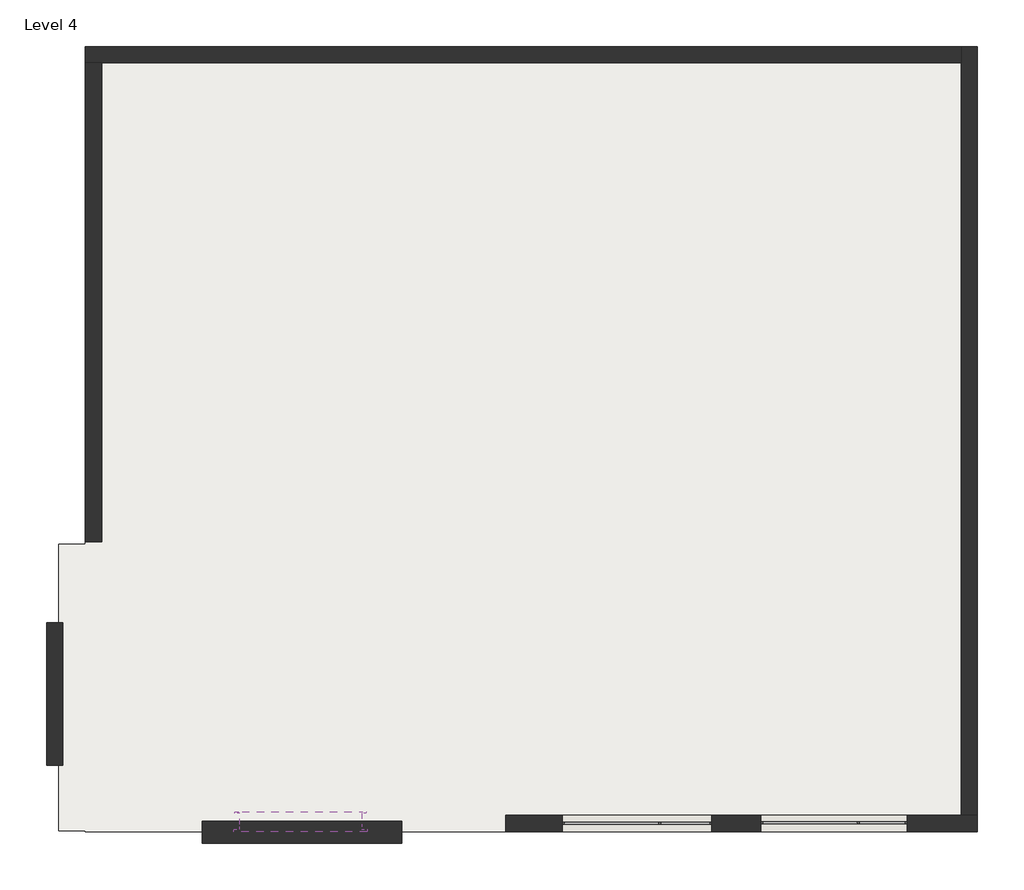
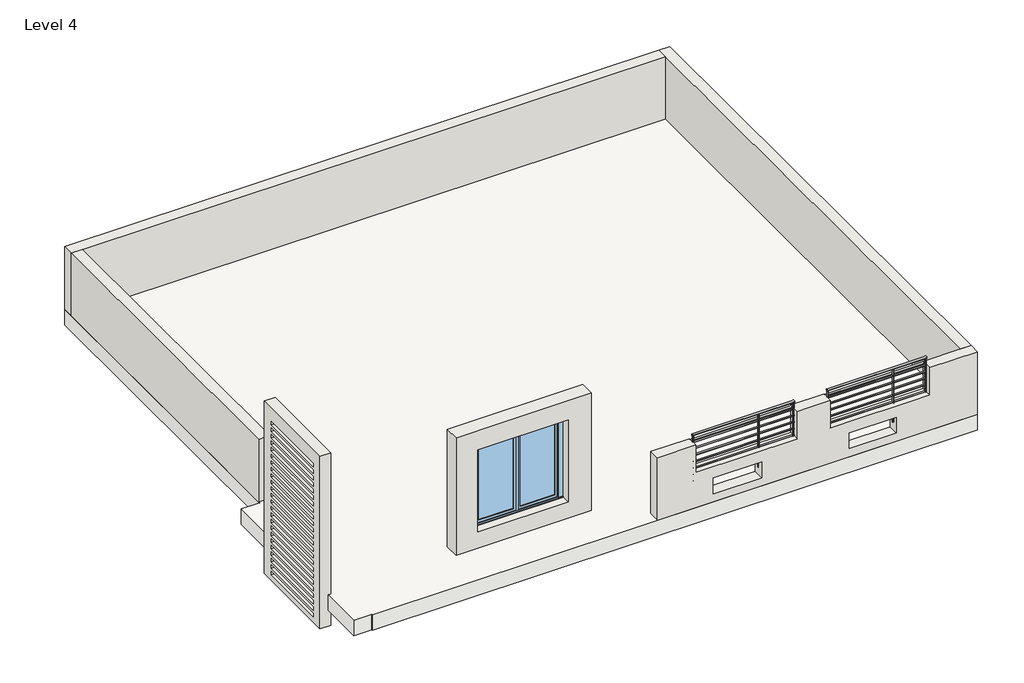
# One storey: 6 walls, 2 railings, 1 roof, 1 window.
"""IFC4 building model written with IfcOpenShell, lengths in millimetres."""

from ifc_helpers import new_model, si_unit, point, frame, frame_2d, origin, place, context, project, spatial, polyline, circle_curve, trimmed, segment, composite_curve, outline, extrude, faceted_brep, transform, mapped, element, save
from components import walls_2_walls_1_3adabfa7, window_514a67b1

model = new_model("IFC4")

# Units and contexts
model_context = context("Model", 3, world=origin())
ifc_project = project(units=[si_unit("LENGTHUNIT", "METRE", prefix="MILLI")], contexts=[model_context])

# Site, building, storey
site = spatial("IfcSite", under=ifc_project)
building = spatial("IfcBuilding", under=site)
storey = spatial("IfcBuildingStorey", under=building, Name="Level 4", Elevation=10972.8)

# Railings
placement = place(None, origin())
element("IfcRailing", 1, ObjectType="Guardrail - Pipe", at=placement, inside=storey, context=model_context, shape_type="SweptSolid", body=[
    extrude(outline(composite_curve([segment(trimmed(circle_curve(frame_2d((1736.4093308, 12477.75)), 19.05), [point((1717.3593308, 12477.75))], [point((1755.4593308, 12477.75))], False, "CARTESIAN"), True, "CONTINUOUS"), segment(trimmed(circle_curve(frame_2d((1736.4093308, 12477.75)), 19.05), [point((1755.4593308, 12477.75))], [point((1717.3593308, 12477.75))], False, "CARTESIAN"), True, "CONTINUOUS")], self_intersect=False)), frame((-4064.538951, 0.0, 0.0), z_axis=(1.0, 0.0, 0.0), x_axis=(0.0, 1.0, 0.0)), (0.0, 0.0, 1.0), 1872.0501462),
    extrude(outline(composite_curve([segment(trimmed(circle_curve(frame_2d((1660.2093308, 12630.15)), 19.05), [point((1641.1593308, 12630.15))], [point((1679.2593308, 12630.15))], False, "CARTESIAN"), True, "CONTINUOUS"), segment(trimmed(circle_curve(frame_2d((1660.2093308, 12630.15)), 19.05), [point((1679.2593308, 12630.15))], [point((1641.1593308, 12630.15))], False, "CARTESIAN"), True, "CONTINUOUS")], self_intersect=False)), frame((-4064.538951, 0.0, 0.0), z_axis=(1.0, 0.0, 0.0), x_axis=(0.0, 1.0, 0.0)), (0.0, 0.0, 1.0), 1872.0501462),
    extrude(outline(composite_curve([segment(trimmed(circle_curve(frame_2d((1660.2093308, 12484.1)), 12.7), [point((1672.9093308, 12484.1))], [point((1647.5093308, 12484.1))], False, "CARTESIAN"), True, "CONTINUOUS"), segment(trimmed(circle_curve(frame_2d((1660.2093308, 12484.1)), 12.7), [point((1647.5093308, 12484.1))], [point((1672.9093308, 12484.1))], False, "CARTESIAN"), True, "CONTINUOUS")], self_intersect=False)), frame((-4064.538951, 0.0, 0.0), z_axis=(1.0, 0.0, 0.0), x_axis=(0.0, 1.0, 0.0)), (0.0, 0.0, 1.0), 1872.0501462),
    extrude(outline(composite_curve([segment(trimmed(circle_curve(frame_2d((1660.2093308, 12357.1)), 12.7), [point((1672.9093308, 12357.1))], [point((1647.5093308, 12357.1))], False, "CARTESIAN"), True, "CONTINUOUS"), segment(trimmed(circle_curve(frame_2d((1660.2093308, 12357.1)), 12.7), [point((1647.5093308, 12357.1))], [point((1672.9093308, 12357.1))], False, "CARTESIAN"), True, "CONTINUOUS")], self_intersect=False)), frame((-4064.538951, 0.0, 0.0), z_axis=(1.0, 0.0, 0.0), x_axis=(0.0, 1.0, 0.0)), (0.0, 0.0, 1.0), 1872.0501462),
    extrude(outline(composite_curve([segment(trimmed(circle_curve(frame_2d((1660.2093308, 12230.1)), 12.7), [point((1672.9093308, 12230.1))], [point((1647.5093308, 12230.1))], False, "CARTESIAN"), True, "CONTINUOUS"), segment(trimmed(circle_curve(frame_2d((1660.2093308, 12230.1)), 12.7), [point((1647.5093308, 12230.1))], [point((1672.9093308, 12230.1))], False, "CARTESIAN"), True, "CONTINUOUS")], self_intersect=False)), frame((-4064.538951, 0.0, 0.0), z_axis=(1.0, 0.0, 0.0), x_axis=(0.0, 1.0, 0.0)), (0.0, 0.0, 1.0), 1872.0501462),
    extrude(outline(composite_curve([segment(trimmed(circle_curve(frame_2d((1660.2093308, 12103.1)), 12.7), [point((1672.9093308, 12103.1))], [point((1647.5093308, 12103.1))], False, "CARTESIAN"), True, "CONTINUOUS"), segment(trimmed(circle_curve(frame_2d((1660.2093308, 12103.1)), 12.7), [point((1647.5093308, 12103.1))], [point((1672.9093308, 12103.1))], False, "CARTESIAN"), True, "CONTINUOUS")], self_intersect=False)), frame((-4064.538951, 0.0, 0.0), z_axis=(1.0, 0.0, 0.0), x_axis=(0.0, 1.0, 0.0)), (0.0, 0.0, 1.0), 1872.0501462),
    extrude(outline(composite_curve([segment(trimmed(circle_curve(frame_2d((1660.2093308, 11976.1)), 12.7), [point((1672.9093308, 11976.1))], [point((1647.5093308, 11976.1))], False, "CARTESIAN"), True, "CONTINUOUS"), segment(trimmed(circle_curve(frame_2d((1660.2093308, 11976.1)), 12.7), [point((1647.5093308, 11976.1))], [point((1672.9093308, 11976.1))], False, "CARTESIAN"), True, "CONTINUOUS")], self_intersect=False)), frame((-4064.538951, 0.0, 0.0), z_axis=(1.0, 0.0, 0.0), x_axis=(0.0, 1.0, 0.0)), (0.0, 0.0, 1.0), 1872.0501462),
    extrude(outline(composite_curve([segment(trimmed(circle_curve(frame_2d((1660.2093308, 11849.1)), 12.7), [point((1672.9093308, 11849.1))], [point((1647.5093308, 11849.1))], False, "CARTESIAN"), True, "CONTINUOUS"), segment(trimmed(circle_curve(frame_2d((1660.2093308, 11849.1)), 12.7), [point((1647.5093308, 11849.1))], [point((1672.9093308, 11849.1))], False, "CARTESIAN"), True, "CONTINUOUS")], self_intersect=False)), frame((-4064.538951, 0.0, 0.0), z_axis=(1.0, 0.0, 0.0), x_axis=(0.0, 1.0, 0.0)), (0.0, 0.0, 1.0), 1872.0501462),
    extrude(outline(composite_curve([segment(trimmed(circle_curve(frame_2d((1660.2093308, 11722.1)), 12.7), [point((1672.9093308, 11722.1))], [point((1647.5093308, 11722.1))], False, "CARTESIAN"), True, "CONTINUOUS"), segment(trimmed(circle_curve(frame_2d((1660.2093308, 11722.1)), 12.7), [point((1647.5093308, 11722.1))], [point((1672.9093308, 11722.1))], False, "CARTESIAN"), True, "CONTINUOUS")], self_intersect=False)), frame((-4064.538951, 0.0, 0.0), z_axis=(1.0, 0.0, 0.0), x_axis=(0.0, 1.0, 0.0)), (0.0, 0.0, 1.0), 1872.0501462),
    extrude(outline(composite_curve([segment(trimmed(circle_curve(frame_2d((-2845.338951, 1660.2093308)), 12.7), [point((-2845.338951, 1672.9093308))], [point((-2845.338951, 1647.5093308))], False, "CARTESIAN"), True, "CONTINUOUS"), segment(trimmed(circle_curve(frame_2d((-2845.338951, 1660.2093308)), 12.7), [point((-2845.338951, 1647.5093308))], [point((-2845.338951, 1672.9093308))], False, "CARTESIAN"), True, "CONTINUOUS")], self_intersect=False)), frame((0.0, 0.0, 11582.4), z_axis=(0.0, 0.0, 1.0), x_axis=(1.0, 0.0, 0.0)), (0.0, 0.0, 1.0), 1028.7),
    extrude(outline(composite_curve([segment(trimmed(circle_curve(frame_2d((-2205.1888049, 1660.2093308)), 12.7), [point((-2205.1888049, 1672.9093308))], [point((-2205.1888049, 1647.5093308))], False, "CARTESIAN"), True, "CONTINUOUS"), segment(trimmed(circle_curve(frame_2d((-2205.1888049, 1660.2093308)), 12.7), [point((-2205.1888049, 1647.5093308))], [point((-2205.1888049, 1672.9093308))], False, "CARTESIAN"), True, "CONTINUOUS")], self_intersect=False)), frame((0.0, 0.0, 11582.4), z_axis=(0.0, 0.0, 1.0), x_axis=(1.0, 0.0, 0.0)), (0.0, 0.0, 1.0), 1028.7),
    extrude(outline(composite_curve([segment(trimmed(circle_curve(frame_2d((-4051.838951, 1660.2093308)), 12.7), [point((-4051.838951, 1672.9093308))], [point((-4051.838951, 1647.5093308))], False, "CARTESIAN"), True, "CONTINUOUS"), segment(trimmed(circle_curve(frame_2d((-4051.838951, 1660.2093308)), 12.7), [point((-4051.838951, 1647.5093308))], [point((-4051.838951, 1672.9093308))], False, "CARTESIAN"), True, "CONTINUOUS")], self_intersect=False)), frame((0.0, 0.0, 11582.4), z_axis=(0.0, 0.0, 1.0), x_axis=(1.0, 0.0, 0.0)), (0.0, 0.0, 1.0), 1028.7),
])
element("IfcRailing", 2, ObjectType="Guardrail - Pipe", at=placement, inside=storey, context=model_context, shape_type="SweptSolid", body=[
    extrude(outline(composite_curve([segment(trimmed(circle_curve(frame_2d((1742.0864664, 12477.75)), 19.05), [point((1723.0364664, 12477.75))], [point((1761.1364664, 12477.75))], False, "CARTESIAN"), True, "CONTINUOUS"), segment(trimmed(circle_curve(frame_2d((1742.0864664, 12477.75)), 19.05), [point((1761.1364664, 12477.75))], [point((1723.0364664, 12477.75))], False, "CARTESIAN"), True, "CONTINUOUS")], self_intersect=False)), frame((-1582.8888049, 0.0, 0.0), z_axis=(1.0, 0.0, 0.0), x_axis=(0.0, 1.0, 0.0)), (0.0, 0.0, 1.0), 1827.3417832),
    extrude(outline(composite_curve([segment(trimmed(circle_curve(frame_2d((1665.8864664, 12630.15)), 19.05), [point((1646.8364664, 12630.15))], [point((1684.9364664, 12630.15))], False, "CARTESIAN"), True, "CONTINUOUS"), segment(trimmed(circle_curve(frame_2d((1665.8864664, 12630.15)), 19.05), [point((1684.9364664, 12630.15))], [point((1646.8364664, 12630.15))], False, "CARTESIAN"), True, "CONTINUOUS")], self_intersect=False)), frame((-1582.8888049, 0.0, 0.0), z_axis=(1.0, 0.0, 0.0), x_axis=(0.0, 1.0, 0.0)), (0.0, 0.0, 1.0), 1827.3417832),
    extrude(outline(composite_curve([segment(trimmed(circle_curve(frame_2d((1665.8864664, 12484.1)), 12.7), [point((1678.5864664, 12484.1))], [point((1653.1864664, 12484.1))], False, "CARTESIAN"), True, "CONTINUOUS"), segment(trimmed(circle_curve(frame_2d((1665.8864664, 12484.1)), 12.7), [point((1653.1864664, 12484.1))], [point((1678.5864664, 12484.1))], False, "CARTESIAN"), True, "CONTINUOUS")], self_intersect=False)), frame((-1582.8888049, 0.0, 0.0), z_axis=(1.0, 0.0, 0.0), x_axis=(0.0, 1.0, 0.0)), (0.0, 0.0, 1.0), 1827.3417832),
    extrude(outline(composite_curve([segment(trimmed(circle_curve(frame_2d((1665.8864664, 12357.1)), 12.7), [point((1678.5864664, 12357.1))], [point((1653.1864664, 12357.1))], False, "CARTESIAN"), True, "CONTINUOUS"), segment(trimmed(circle_curve(frame_2d((1665.8864664, 12357.1)), 12.7), [point((1653.1864664, 12357.1))], [point((1678.5864664, 12357.1))], False, "CARTESIAN"), True, "CONTINUOUS")], self_intersect=False)), frame((-1582.8888049, 0.0, 0.0), z_axis=(1.0, 0.0, 0.0), x_axis=(0.0, 1.0, 0.0)), (0.0, 0.0, 1.0), 1827.3417832),
    extrude(outline(composite_curve([segment(trimmed(circle_curve(frame_2d((1665.8864664, 12230.1)), 12.7), [point((1678.5864664, 12230.1))], [point((1653.1864664, 12230.1))], False, "CARTESIAN"), True, "CONTINUOUS"), segment(trimmed(circle_curve(frame_2d((1665.8864664, 12230.1)), 12.7), [point((1653.1864664, 12230.1))], [point((1678.5864664, 12230.1))], False, "CARTESIAN"), True, "CONTINUOUS")], self_intersect=False)), frame((-1582.8888049, 0.0, 0.0), z_axis=(1.0, 0.0, 0.0), x_axis=(0.0, 1.0, 0.0)), (0.0, 0.0, 1.0), 1827.3417832),
    extrude(outline(composite_curve([segment(trimmed(circle_curve(frame_2d((1665.8864664, 12103.1)), 12.7), [point((1678.5864664, 12103.1))], [point((1653.1864664, 12103.1))], False, "CARTESIAN"), True, "CONTINUOUS"), segment(trimmed(circle_curve(frame_2d((1665.8864664, 12103.1)), 12.7), [point((1653.1864664, 12103.1))], [point((1678.5864664, 12103.1))], False, "CARTESIAN"), True, "CONTINUOUS")], self_intersect=False)), frame((-1582.8888049, 0.0, 0.0), z_axis=(1.0, 0.0, 0.0), x_axis=(0.0, 1.0, 0.0)), (0.0, 0.0, 1.0), 1827.3417832),
    extrude(outline(composite_curve([segment(trimmed(circle_curve(frame_2d((1665.8864664, 11976.1)), 12.7), [point((1678.5864664, 11976.1))], [point((1653.1864664, 11976.1))], False, "CARTESIAN"), True, "CONTINUOUS"), segment(trimmed(circle_curve(frame_2d((1665.8864664, 11976.1)), 12.7), [point((1653.1864664, 11976.1))], [point((1678.5864664, 11976.1))], False, "CARTESIAN"), True, "CONTINUOUS")], self_intersect=False)), frame((-1582.8888049, 0.0, 0.0), z_axis=(1.0, 0.0, 0.0), x_axis=(0.0, 1.0, 0.0)), (0.0, 0.0, 1.0), 1827.3417832),
    extrude(outline(composite_curve([segment(trimmed(circle_curve(frame_2d((1665.8864664, 11849.1)), 12.7), [point((1678.5864664, 11849.1))], [point((1653.1864664, 11849.1))], False, "CARTESIAN"), True, "CONTINUOUS"), segment(trimmed(circle_curve(frame_2d((1665.8864664, 11849.1)), 12.7), [point((1653.1864664, 11849.1))], [point((1678.5864664, 11849.1))], False, "CARTESIAN"), True, "CONTINUOUS")], self_intersect=False)), frame((-1582.8888049, 0.0, 0.0), z_axis=(1.0, 0.0, 0.0), x_axis=(0.0, 1.0, 0.0)), (0.0, 0.0, 1.0), 1827.3417832),
    extrude(outline(composite_curve([segment(trimmed(circle_curve(frame_2d((1665.8864664, 11722.1)), 12.7), [point((1678.5864664, 11722.1))], [point((1653.1864664, 11722.1))], False, "CARTESIAN"), True, "CONTINUOUS"), segment(trimmed(circle_curve(frame_2d((1665.8864664, 11722.1)), 12.7), [point((1653.1864664, 11722.1))], [point((1678.5864664, 11722.1))], False, "CARTESIAN"), True, "CONTINUOUS")], self_intersect=False)), frame((-1582.8888049, 0.0, 0.0), z_axis=(1.0, 0.0, 0.0), x_axis=(0.0, 1.0, 0.0)), (0.0, 0.0, 1.0), 1827.3417832),
    extrude(outline(composite_curve([segment(trimmed(circle_curve(frame_2d((-363.6888049, 1665.8864664)), 12.7), [point((-363.6888049, 1678.5864664))], [point((-363.6888049, 1653.1864664))], False, "CARTESIAN"), True, "CONTINUOUS"), segment(trimmed(circle_curve(frame_2d((-363.6888049, 1665.8864664)), 12.7), [point((-363.6888049, 1653.1864664))], [point((-363.6888049, 1678.5864664))], False, "CARTESIAN"), True, "CONTINUOUS")], self_intersect=False)), frame((0.0, 0.0, 11582.4), z_axis=(0.0, 0.0, 1.0), x_axis=(1.0, 0.0, 0.0)), (0.0, 0.0, 1.0), 1028.7),
    extrude(outline(composite_curve([segment(trimmed(circle_curve(frame_2d((231.7529784, 1665.8864664)), 12.7), [point((231.7529784, 1678.5864664))], [point((231.7529784, 1653.1864664))], False, "CARTESIAN"), True, "CONTINUOUS"), segment(trimmed(circle_curve(frame_2d((231.7529784, 1665.8864664)), 12.7), [point((231.7529784, 1653.1864664))], [point((231.7529784, 1678.5864664))], False, "CARTESIAN"), True, "CONTINUOUS")], self_intersect=False)), frame((0.0, 0.0, 11582.4), z_axis=(0.0, 0.0, 1.0), x_axis=(1.0, 0.0, 0.0)), (0.0, 0.0, 1.0), 1028.7),
    extrude(outline(composite_curve([segment(trimmed(circle_curve(frame_2d((-1570.1888049, 1665.8864664)), 12.7), [point((-1570.1888049, 1678.5864664))], [point((-1570.1888049, 1653.1864664))], False, "CARTESIAN"), True, "CONTINUOUS"), segment(trimmed(circle_curve(frame_2d((-1570.1888049, 1665.8864664)), 12.7), [point((-1570.1888049, 1653.1864664))], [point((-1570.1888049, 1678.5864664))], False, "CARTESIAN"), True, "CONTINUOUS")], self_intersect=False)), frame((0.0, 0.0, 11582.4), z_axis=(0.0, 0.0, 1.0), x_axis=(1.0, 0.0, 0.0)), (0.0, 0.0, 1.0), 1028.7),
])

# Roof
element("IfcRoof", 3, ObjectType="Generic - 12\"", at=placement, inside=storey, context=model_context, shape_type="SweptSolid", body=[
    extrude(outline(polyline([(-10018.4747472, 11358.0609482), (1122.6002528, 11358.0609482), (1122.6002528, 1553.6609482), (-10019.8638097, 1553.6609482), (-10019.8638097, 1567.9484482), (-10352.5857575, 1567.9484482), (-10352.5857575, 5144.9959854), (-10018.4747472, 5144.9959854), (-10018.4747472, 11358.0609482)])), frame((0.0, 0.0, 10972.8), z_axis=(0.0, 0.0, 1.0), x_axis=(1.0, 0.0, 0.0)), (0.0, 0.0, 1.0), 304.8),
])

# Walls
element("IfcWall", 4, ObjectType="Generic - 8\"", at=placement, inside=storey, context=model_context, shape_type="Brep", body=[
    faceted_brep([(-4770.1997472, 1553.6609482, 11277.6), (1122.6002528, 1553.6609482, 11277.6), (1122.6002528, 1553.6609482, 11963.4), (1122.6002528, 1553.6609482, 12496.8), (244.4529784, 1553.6609482, 12496.8), (244.4529784, 1553.6609482, 11963.4), (-1582.8888049, 1553.6609482, 11963.4), (-1582.8888049, 1553.6609482, 12496.8), (-2192.4888049, 1553.6609482, 12496.8), (-2192.4888049, 1553.6609482, 11963.4), (-4064.538951, 1553.6609482, 11963.4), (-4064.538951, 1553.6609482, 12496.8), (-4770.1997472, 1553.6609482, 12496.8), (-2852.1449663, 1553.6609482, 11741.1892952), (-2852.1449663, 1553.6609482, 11436.3892952), (-3741.1449663, 1553.6609482, 11436.3892952), (-3741.1449663, 1553.6609482, 11741.1892952), (-369.8611252, 1553.6609482, 11741.1892952), (-369.8611252, 1553.6609482, 11436.3892952), (-1235.0084685, 1553.6609482, 11436.3892952), (-1235.0084685, 1553.6609482, 11741.1892952), (-4770.1997472, 1756.8609482, 11277.6), (-4770.1997472, 1756.8609482, 12496.8), (-4064.538951, 1756.8609482, 12496.8), (-4064.538951, 1756.8609482, 11963.4), (-2192.4888049, 1756.8609482, 11963.4), (-2192.4888049, 1756.8609482, 12496.8), (-1582.8888049, 1756.8609482, 12496.8), (-1582.8888049, 1756.8609482, 11963.4), (244.4529784, 1756.8609482, 11963.4), (244.4529784, 1756.8609482, 12496.8), (919.4002528, 1756.8609482, 12496.8), (1122.6002528, 1756.8609482, 12496.8), (1122.6002528, 1756.8609482, 11963.4), (1122.6002528, 1756.8609482, 11277.6), (919.4002528, 1756.8609482, 11277.6), (-2852.1449663, 1756.8609482, 11741.1892952), (-3741.1449663, 1756.8609482, 11741.1892952), (-3741.1449663, 1756.8609482, 11436.3892952), (-2852.1449663, 1756.8609482, 11436.3892952), (-369.8611252, 1756.8609482, 11741.1892952), (-1235.0084685, 1756.8609482, 11741.1892952), (-1235.0084685, 1756.8609482, 11436.3892952), (-369.8611252, 1756.8609482, 11436.3892952)], [[[0, 1, 2, 3, 4, 5, 6, 7, 8, 9, 10, 11, 12], [13, 14, 15, 16], [17, 18, 19, 20]], [[21, 22, 23, 24, 25, 26, 27, 28, 29, 30, 31, 32, 33, 34, 35], [36, 37, 38, 39], [40, 41, 42, 43]], [[1, 0, 21, 35, 34]], [[0, 12, 22, 21]], [[6, 5, 29, 28]], [[7, 6, 28, 27]], [[8, 7, 27, 26]], [[9, 8, 26, 25]], [[10, 9, 25, 24]], [[14, 13, 36, 39]], [[15, 14, 39, 38]], [[16, 15, 38, 37]], [[13, 16, 37, 36]], [[18, 17, 40, 43]], [[19, 18, 43, 42]], [[20, 19, 42, 41]], [[17, 20, 41, 40]], [[4, 3, 32, 31, 30]], [[5, 4, 30, 29]], [[11, 10, 24, 23]], [[12, 11, 23, 22]], [[3, 2, 1, 34, 33, 32]]]),
])
element("IfcWall", 5, ObjectType="Generic - 8\"", at=placement, inside=storey, context=model_context, shape_type="Brep", body=[
    faceted_brep([(1122.6002528, 1756.8609482, 11277.6), (1122.6002528, 11358.0609482, 11277.6), (1122.6002528, 11358.0609482, 12496.8), (1122.6002528, 1756.8609482, 12496.8), (919.4002528, 1756.8609482, 11277.6), (919.4002528, 1756.8609482, 12496.8), (919.4002528, 11154.8609482, 12496.8), (919.4002528, 11358.0609482, 12496.8), (919.4002528, 11358.0609482, 11277.6), (919.4002528, 11154.8609482, 11277.6)], [[[0, 1, 2, 3]], [[4, 5, 6, 7, 8, 9]], [[1, 0, 4, 9, 8]], [[3, 2, 7, 6, 5]], [[0, 3, 5, 4]], [[2, 1, 8, 7]]]),
])
element("IfcWall", 6, ObjectType="Generic - 8\"", at=placement, inside=storey, context=model_context, shape_type="Brep", body=[
    faceted_brep([(919.4002528, 11358.0609482, 11277.6), (-10018.4747472, 11358.0609482, 11277.6), (-10018.4747472, 11358.0609482, 12496.8), (919.4002528, 11358.0609482, 12496.8), (919.4002528, 11154.8609482, 11277.6), (919.4002528, 11154.8609482, 12496.8), (-9815.2747472, 11154.8609482, 12496.8), (-10018.4747472, 11154.8609482, 12496.8), (-10018.4747472, 11154.8609482, 11277.6), (-9815.2747472, 11154.8609482, 11277.6)], [[[0, 1, 2, 3]], [[4, 5, 6, 7, 8, 9]], [[1, 0, 4, 9, 8]], [[3, 2, 7, 6, 5]], [[0, 3, 5, 4]], [[2, 1, 8, 7]]]),
])
element("IfcWall", 7, ObjectType="Generic - 8\"", at=placement, inside=storey, context=model_context, shape_type="Brep", body=[
    faceted_brep([(-10018.4747472, 11154.8609482, 11277.6), (-10018.4747472, 5306.9209854, 11277.6), (-10018.4747472, 5179.9209854, 11277.6), (-10018.4747472, 5174.7484482, 11277.6), (-10018.4747472, 5174.7484482, 12496.8), (-10018.4747472, 11154.8609482, 12496.8), (-9815.2747472, 11154.8609482, 11277.6), (-9815.2747472, 11154.8609482, 12496.8), (-9815.2747472, 5174.7484482, 12496.8), (-9815.2747472, 5174.7484482, 11277.6)], [[[0, 1, 2, 3, 4, 5]], [[6, 7, 8, 9]], [[3, 2, 1, 0, 6, 9]], [[5, 4, 8, 7]], [[0, 5, 7, 6]], [[4, 3, 9, 8]]]),
])
element("IfcWall", 8, ObjectType="Generic - 8\"", at=placement, inside=storey, context=model_context, shape_type="SweptSolid", body=[
    extrude(outline(polyline([(4162.4454783, 10668.0), (2382.8579783, 10668.0), (2382.8579783, 14023.1950228), (4162.4454783, 14023.1950228), (4162.4454783, 10668.0)]), holes=[polyline([(3937.4533381, 13762.2542182), (2591.2533381, 13762.2542182), (2591.2533381, 13698.7542182), (3937.4533381, 13698.7542182), (3937.4533381, 13762.2542182)]), polyline([(3937.4533381, 13635.2542182), (2591.2533381, 13635.2542182), (2591.2533381, 13571.7542182), (3937.4533381, 13571.7542182), (3937.4533381, 13635.2542182)]), polyline([(3937.4533381, 13508.2542182), (2591.2533381, 13508.2542182), (2591.2533381, 13444.7542182), (3937.4533381, 13444.7542182), (3937.4533381, 13508.2542182)]), polyline([(3937.4533381, 13381.2542182), (2591.2533381, 13381.2542182), (2591.2533381, 13317.7542182), (3937.4533381, 13317.7542182), (3937.4533381, 13381.2542182)]), polyline([(3937.4533381, 13254.2542182), (2591.2533381, 13254.2542182), (2591.2533381, 13190.7542182), (3937.4533381, 13190.7542182), (3937.4533381, 13254.2542182)]), polyline([(3937.4533381, 13127.2542182), (2591.2533381, 13127.2542182), (2591.2533381, 13063.7542182), (3937.4533381, 13063.7542182), (3937.4533381, 13127.2542182)]), polyline([(3937.4533381, 13000.2542182), (2591.2533381, 13000.2542182), (2591.2533381, 12936.7542182), (3937.4533381, 12936.7542182), (3937.4533381, 13000.2542182)]), polyline([(3937.4533381, 12873.2542182), (2591.2533381, 12873.2542182), (2591.2533381, 12809.7542182), (3937.4533381, 12809.7542182), (3937.4533381, 12873.2542182)]), polyline([(3937.4533381, 12746.2542182), (2591.2533381, 12746.2542182), (2591.2533381, 12682.7542182), (3937.4533381, 12682.7542182), (3937.4533381, 12746.2542182)]), polyline([(3937.4533381, 12619.2542182), (2591.2533381, 12619.2542182), (2591.2533381, 12555.7542182), (3937.4533381, 12555.7542182), (3937.4533381, 12619.2542182)]), polyline([(3937.4533381, 12492.2542182), (2591.2533381, 12492.2542182), (2591.2533381, 12428.7542182), (3937.4533381, 12428.7542182), (3937.4533381, 12492.2542182)]), polyline([(3937.4533381, 12365.2542182), (2591.2533381, 12365.2542182), (2591.2533381, 12301.7542182), (3937.4533381, 12301.7542182), (3937.4533381, 12365.2542182)]), polyline([(3937.4533381, 12238.2542182), (2591.2533381, 12238.2542182), (2591.2533381, 12174.7542182), (3937.4533381, 12174.7542182), (3937.4533381, 12238.2542182)]), polyline([(3937.4533381, 12111.2542182), (2591.2533381, 12111.2542182), (2591.2533381, 12047.7542182), (3937.4533381, 12047.7542182), (3937.4533381, 12111.2542182)]), polyline([(3937.4533381, 11984.2542182), (2591.2533381, 11984.2542182), (2591.2533381, 11920.7542182), (3937.4533381, 11920.7542182), (3937.4533381, 11984.2542182)]), polyline([(3937.4533381, 11857.2542182), (2591.2533381, 11857.2542182), (2591.2533381, 11793.7542182), (3937.4533381, 11793.7542182), (3937.4533381, 11857.2542182)]), polyline([(3937.4533381, 11730.2542182), (2591.2533381, 11730.2542182), (2591.2533381, 11666.7542182), (3937.4533381, 11666.7542182), (3937.4533381, 11730.2542182)]), polyline([(3937.4533381, 11603.2542182), (2591.2533381, 11603.2542182), (2591.2533381, 11539.7542182), (3937.4533381, 11539.7542182), (3937.4533381, 11603.2542182)]), polyline([(3937.4533381, 11476.2542182), (2591.2533381, 11476.2542182), (2591.2533381, 11412.7542182), (3937.4533381, 11412.7542182), (3937.4533381, 11476.2542182)]), polyline([(3937.4533381, 11349.2542182), (2591.2533381, 11349.2542182), (2591.2533381, 11285.7542182), (3937.4533381, 11285.7542182), (3937.4533381, 11349.2542182)]), polyline([(3937.4533381, 11222.2542182), (2591.2533381, 11222.2542182), (2591.2533381, 11158.7542182), (3937.4533381, 11158.7542182), (3937.4533381, 11222.2542182)]), polyline([(3937.4533381, 11095.2542182), (2591.2533381, 11095.2542182), (2591.2533381, 11031.7542182), (3937.4533381, 11031.7542182), (3937.4533381, 11095.2542182)]), polyline([(3937.4533381, 10968.2542182), (2591.2533381, 10968.2542182), (2591.2533381, 10904.7542182), (3937.4533381, 10904.7542182), (3937.4533381, 10968.2542182)]), polyline([(3937.4533381, 10841.2542182), (2591.2533381, 10841.2542182), (2591.2533381, 10777.7542182), (3937.4533381, 10777.7542182), (3937.4533381, 10841.2542182)])]), frame((-10502.5452839, 0.0, 0.0), z_axis=(1.0, 0.0, 0.0), x_axis=(0.0, 1.0, 0.0)), (0.0, 0.0, 1.0), 203.2),
])
walls_2_walls_1_shape = walls_2_walls_1_3adabfa7(model_context)
element("IfcWall", 9, ObjectType="Walls 2 : Walls 1", at=placement, inside=storey, context=model_context, shape_type="MappedRepresentation", body=[
    mapped(walls_2_walls_1_shape, transform((0.0, 0.0, 0.0), x_axis=(1.0, 0.0, 0.0), y_axis=(0.0, 1.0, 0.0), z_axis=(0.0, 0.0, 1.0))),
])

# Window
window_shape = window_514a67b1(model_context)
element("IfcWindow", 10, ObjectType="Casement Dbl with Trim.0001 : 60\" x 60\"", at=placement, inside=storey, context=model_context, shape_type="MappedRepresentation", body=[
    mapped(window_shape, transform((-7329.9857575, 1701.2984482, 11417.4181256), x_axis=(-1.0, 0.0, 0.0), y_axis=(0.0, -1.0, 0.0), z_axis=(0.0, 0.0, 1.0))),
])

save(model, "model.ifc")

# Revit data of these elements
# Type "Guardrail - Pipe"
#   Assembly Code = "C2010400"
#   built-in parameter 1008612 = 0.0416667 (stored number, unit not read)
#   built-in parameter 1008611 = 0.0833333 (stored number, unit not read)
#   built-in parameter 1008609 = 4 (stored number, unit not read)
#   built-in parameter 1008604 = 0.166667 (stored number, unit not read)
#   built-in parameter 1008603 = 0.166667 (stored number, unit not read)
#   Railing Height = 3' - 6"
#   built-in parameter 1008630 = 2
#   built-in parameter 1008610 = 1
#   built-in parameter 1008605 = 1
#   built-in parameter 1008618 = Baluster - Round : 1"
# Type "Generic - 12\""
#   Assembly Code = "B1020"
#   Layers, outside or top first: 1' - 0" no material (function 1)
# Type "Generic - 8\""
#   Assembly Code = "B2010"
#   Layers, outside or top first: 0' - 8" no material (function 1)
# Type "Casement Dbl with Trim.0001 : 60\" x 60\""
#   Type Mark = "10"
#   Construction Type Id = "GSP4R"
#   Assembly Code = "B2020100"
#   Analytic Construction = "1/8 in Pilkington single glazing"
#   Visual Light Transmittance = 0.9
#   Solar Heat Gain Coefficient = 0.78
#   Heat Transfer Coefficient (U) = 0.6496 BTU/(h·ft²·°F)
#   Height = 5' - 0"
#   Default Sill Height = 3' - 0"
#   Trim Projection - Ext. = 0' - 0 1/2"
#   Trim Projection - Int. = 0' - 0 3/4"
#   Trim Width - Exterior = 0' - 3 1/2"
#   Trim Width - Interior = 0' - 3 1/2"
#   Width = 5' - 0"
#   Window Inset = 0' - 0 3/4"
#   Define Thermal Properties by = 1
#   Glass Pane Material = Glass
#   Sash Material = Sash
#   Trim Exterior Material = Trim
#   Trim Interior Material = Trim
#   Wall Closure = (empty or 0)
# Elements 1, 2 (IfcRailing, "Guardrail - Pipe")
#   built-in parameter 1008621 = 2 (stored number, unit not read)
#   Phase Created = New Construction
# Element 3 (IfcRoof, "Generic - 12\"")
#   built-in parameter 1001705 = 37 (stored number, unit not read)
#   built-in parameter 1001710 = 33615
#   Phase Created = New Construction
#   Materials on its faces: "Default Roof"
# Elements 4, 5, 6, 7 (IfcWall, "Generic - 8\"")
#   built-in parameter 1001111 = 1' - 0"
#   Top Offset = 0' - 0"
#   Base Offset = 1' - 0"
#   Unconnected Height = 4' - 0"
#   wall height = 4' - 0"
#   Phase Created = New Construction
#   Base Constraint = Level 4
#   Materials on its faces: "Default Wall"
# Element 8 (IfcWall, "Generic - 8\"")
#   built-in parameter 1001111 = -1' - 0"
#   Top Offset = 0' - 0"
#   Base Offset = -1' - 0"
#   Unconnected Height = 11' - 0.09429"
#   wall height = 11' - 0.09429"
#   Phase Created = New Construction
#   Base Constraint = Level 4
#   Materials on its faces: "Default Wall"
# Element 9 (IfcWall, "Walls 2 : Walls 1")
#   Phase Created = New Construction
#   Materials on its faces: "Default Wall"
# Element 10 (IfcWindow, "Casement Dbl with Trim.0001 : 60\" x 60\"")
#   Mark = "3"
#   Phase Created = New Construction
#   Materials on its faces: "Sash", "Trim", "Glass"
# Materials
#   "Glass": class "Glass", colour RGB 0 128 192, transparency 0.75, Description = "Soda Lime Glass", Cost = 0
#   "Sash": class "Wood", colour RGB 224 178 126, transparency 0
#   "Trim": class "Wood", colour RGB 224 178 126, transparency 0
#   "Default Roof": colour RGB 88 101 114, transparency 0
#   "Default Wall": colour RGB 128 128 128, transparency 0
